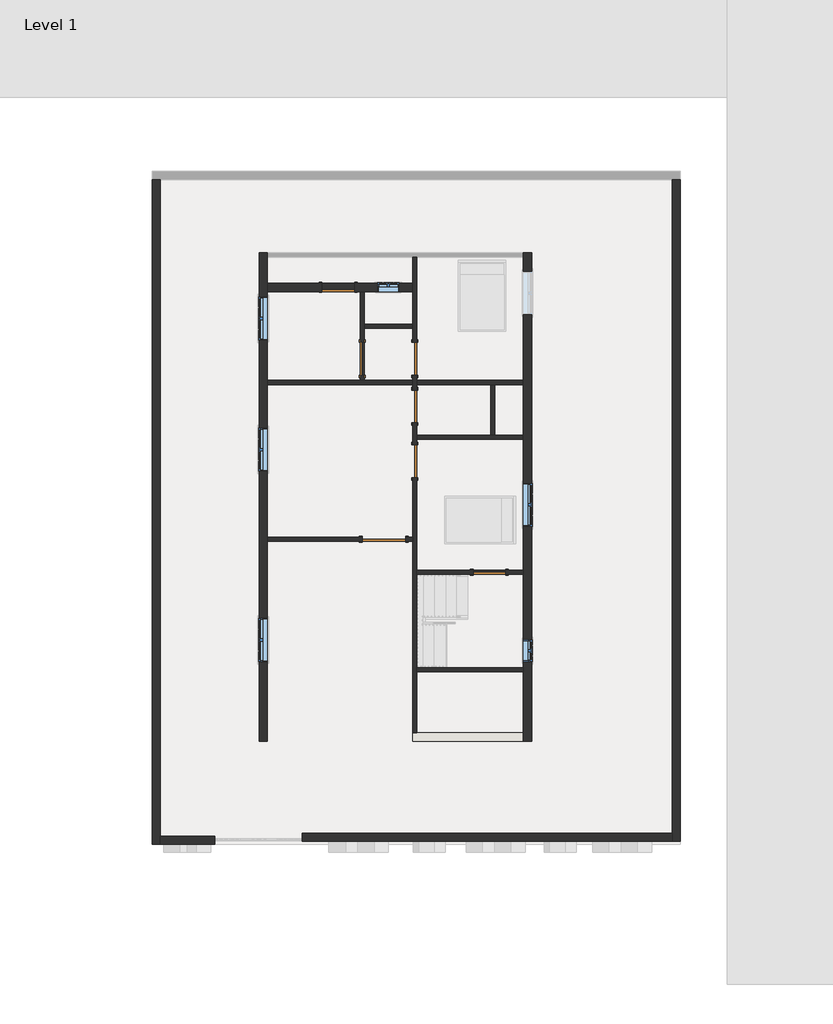
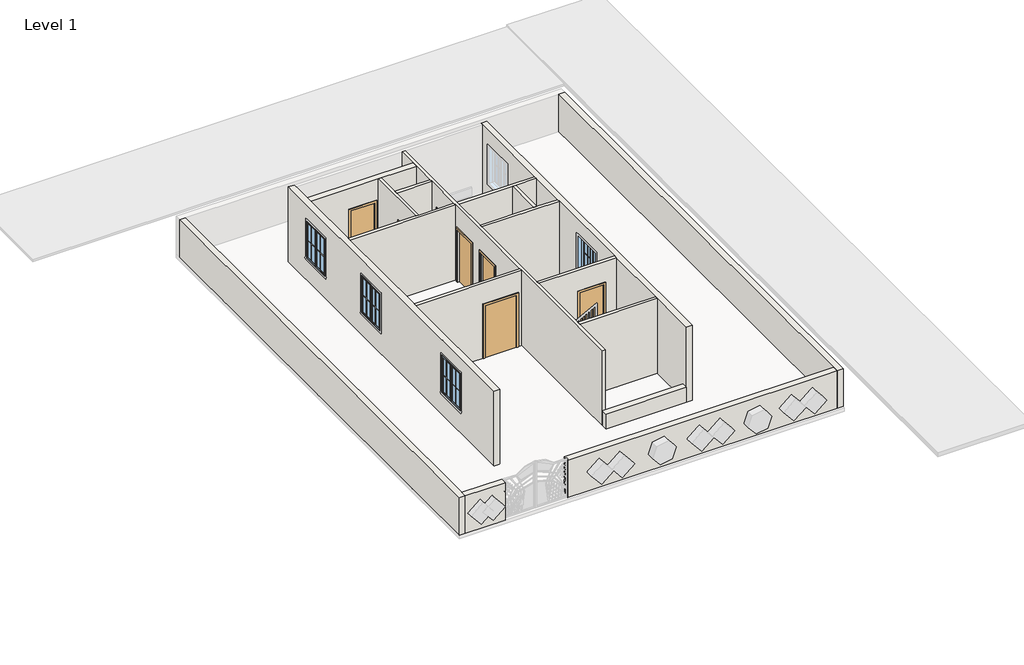
# One storey, part 1 of 7: 26 walls, 7 doors, 7 windows.
"""IFC4 building model written with IfcOpenShell, lengths in millimetres."""

from ifc_helpers import new_model, si_unit, frame, origin, origin_with_axes, place, context, project, spatial, polyline, outline, extrude, faceted_brep, transform, mapped, element, save
from components import door_a90ba1ad, door_e5f9f3c4, door_305aa2a5, door_6ea84ebe, window_c417fced, window_8377141f

model = new_model("IFC4")

# Units and contexts
model_context = context("Model", 3, world=origin())
ifc_project = project(units=[si_unit("LENGTHUNIT", "METRE", prefix="MILLI")], contexts=[model_context])

# Site, building, storey
site = spatial("IfcSite", under=ifc_project)
building = spatial("IfcBuilding", under=site)
storey = spatial("IfcBuildingStorey", under=building, Name="Level 1", Elevation=0.0)

# Doors
placement = place(None, origin())
door_shape = door_a90ba1ad(model_context)
element("IfcDoor", 1, ObjectType="Single-Flush : 36\" x 84\"", at=placement, inside=storey, context=model_context, shape_type="MappedRepresentation", body=[
    mapped(door_shape, transform((3479.8, 13512.8, 0.0), x_axis=(1.0, 0.0, 0.0), y_axis=(0.0, 1.0, 0.0), z_axis=(0.0, 0.0, 1.0))),
])
door_2_shape = door_e5f9f3c4(model_context)
element("IfcDoor", 2, ObjectType="Single-Flush : 36\" x 84\"", at=placement, inside=storey, context=model_context, shape_type="MappedRepresentation", body=[
    mapped(door_2_shape, transform((5619.75, 11518.9, 0.0), x_axis=(0.0, -1.0, 0.0), y_axis=(1.0, 0.0, 0.0), z_axis=(0.0, 0.0, 1.0))),
])
element("IfcDoor", 3, ObjectType="Single-Flush : 36\" x 84\"", at=placement, inside=storey, context=model_context, shape_type="MappedRepresentation", body=[
    mapped(door_2_shape, transform((7708.9, 5543.55, 0.0), x_axis=(-1.0, 0.0, 0.0), y_axis=(0.0, -1.0, 0.0), z_axis=(0.0, 0.0, 1.0))),
])
door_3_shape = door_305aa2a5(model_context)
element("IfcDoor", 4, ObjectType="Single-Flush : 36\" x 84\"", at=placement, inside=storey, context=model_context, shape_type="MappedRepresentation", body=[
    mapped(door_3_shape, transform((4146.55, 11518.9, 0.0), x_axis=(0.0, -1.0, 0.0), y_axis=(1.0, 0.0, 0.0), z_axis=(0.0, 0.0, 1.0))),
])
element("IfcDoor", 5, ObjectType="Single-Flush : 36\" x 84\"", at=placement, inside=storey, context=model_context, shape_type="MappedRepresentation", body=[
    mapped(door_3_shape, transform((5619.75, 10185.4, 0.0), x_axis=(0.0, 1.0, 0.0), y_axis=(-1.0, 0.0, 0.0), z_axis=(0.0, 0.0, 1.0))),
])
element("IfcDoor", 6, ObjectType="Single-Flush : 36\" x 84\"", at=placement, inside=storey, context=model_context, shape_type="MappedRepresentation", body=[
    mapped(door_3_shape, transform((5619.75, 8648.7, 0.0), x_axis=(0.0, 1.0, 0.0), y_axis=(-1.0, 0.0, 0.0), z_axis=(0.0, 0.0, 1.0))),
])
door_4_shape = door_6ea84ebe(model_context)
element("IfcDoor", 7, ObjectType="Single-Flush : 48\" x 84\"", at=placement, inside=storey, context=model_context, shape_type="MappedRepresentation", body=[
    mapped(door_4_shape, transform((4756.15, 6470.65, 0.0), x_axis=(-1.0, 0.0, 0.0), y_axis=(0.0, -1.0, 0.0), z_axis=(0.0, 0.0, 1.0))),
])

# Walls
element("IfcWall", 8, ObjectType="Generic - 5\"", at=placement, inside=storey, context=model_context, shape_type="Brep", body=[
    faceted_brep([(5562.6, 9728.2, 0.0), (5562.6, 9105.9, 0.0), (5562.6, 9105.9, 2133.6), (5562.6, 8191.5, 2133.6), (5562.6, 8191.5, 0.0), (5562.6, 6527.8, 0.0), (5562.6, 6413.5, 0.0), (5562.6, 1047.75, 0.0), (5562.6, 1047.75, 609.6), (5562.6, 1047.75, 3048.0), (5562.6, 6413.5, 3048.0), (5562.6, 6527.8, 3048.0), (5562.6, 10795.0, 3048.0), (5562.6, 10909.3, 3048.0), (5562.6, 12369.8, 3048.0), (5562.6, 12484.1, 3048.0), (5562.6, 13398.5, 3048.0), (5562.6, 13627.1, 3048.0), (5562.6, 14363.7, 3048.0), (5562.6, 14363.7, 0.0), (5562.6, 13627.1, 0.0), (5562.6, 13398.5, 0.0), (5562.6, 12484.1, 0.0), (5562.6, 12369.8, 0.0), (5562.6, 11976.1, 0.0), (5562.6, 11976.1, 2133.6), (5562.6, 11061.7, 2133.6), (5562.6, 11061.7, 0.0), (5562.6, 10909.3, 0.0), (5562.6, 10795.0, 0.0), (5562.6, 10642.6, 0.0), (5562.6, 10642.6, 2133.6), (5562.6, 9728.2, 2133.6), (5676.9, 9105.9, 2133.6), (5676.9, 9105.9, 0.0), (5676.9, 9258.3, 0.0), (5676.9, 9372.6, 0.0), (5676.9, 9728.2, 0.0), (5676.9, 9728.2, 2133.6), (5676.9, 10642.6, 2133.6), (5676.9, 10642.6, 0.0), (5676.9, 10795.0, 0.0), (5676.9, 10909.3, 0.0), (5676.9, 11061.7, 0.0), (5676.9, 11061.7, 2133.6), (5676.9, 11976.1, 2133.6), (5676.9, 11976.1, 0.0), (5676.9, 14363.7, 0.0), (5676.9, 14363.7, 3048.0), (5676.9, 10909.3, 3048.0), (5676.9, 10795.0, 3048.0), (5676.9, 9372.6, 3048.0), (5676.9, 9258.3, 3048.0), (5676.9, 5600.7, 3048.0), (5676.9, 5486.4, 3048.0), (5676.9, 2870.2, 3048.0), (5676.9, 2755.9, 3048.0), (5676.9, 1047.75, 3048.0), (5676.9, 1047.75, 0.0), (5676.9, 2755.9, 0.0), (5676.9, 2870.2, 0.0), (5676.9, 5486.4, 0.0), (5676.9, 5600.7, 0.0), (5676.9, 8191.5, 0.0), (5676.9, 8191.5, 2133.6)], [[[0, 1, 2, 3, 4, 5, 6, 7, 8, 9, 10, 11, 12, 13, 14, 15, 16, 17, 18, 19, 20, 21, 22, 23, 24, 25, 26, 27, 28, 29, 30, 31, 32]], [[33, 34, 35, 36, 37, 38, 39, 40, 41, 42, 43, 44, 45, 46, 47, 48, 49, 50, 51, 52, 53, 54, 55, 56, 57, 58, 59, 60, 61, 62, 63, 64]], [[24, 23, 22, 21, 20, 19, 47, 46]], [[43, 42, 41, 40, 30, 29, 28, 27]], [[37, 36, 35, 34, 1, 0]], [[63, 62, 61, 60, 59, 58, 7, 6, 5, 4]], [[18, 17, 16, 15, 14, 13, 12, 11, 10, 9, 57, 56, 55, 54, 53, 52, 51, 50, 49, 48]], [[19, 18, 48, 47]], [[44, 43, 27, 26]], [[45, 44, 26, 25]], [[46, 45, 25, 24]], [[31, 30, 40, 39]], [[32, 31, 39, 38]], [[0, 32, 38, 37]], [[2, 1, 34, 33]], [[3, 2, 33, 64]], [[4, 3, 64, 63]], [[9, 8, 7, 58, 57]]]),
])
element("IfcWall", 9, ObjectType="Generic - 5\"", at=placement, inside=storey, context=model_context, shape_type="SweptSolid", body=[
    extrude(outline(polyline([(0.0, 5676.9), (0.0, 7251.7), (2133.6, 7251.7), (2133.6, 8166.1), (0.0, 8166.1), (0.0, 8661.4), (3048.0, 8661.4), (3048.0, 5676.9), (0.0, 5676.9)])), frame((0.0, 5486.4, 0.0), z_axis=(0.0, 1.0, 0.0), x_axis=(0.0, 0.0, 1.0)), (0.0, 0.0, 1.0), 114.3),
])
element("IfcWall", 10, ObjectType="Generic - 5\"", at=placement, inside=storey, context=model_context, shape_type="SweptSolid", body=[
    extrude(outline(polyline([(0.0, 1498.6), (0.0, 4146.55), (2133.6, 4146.55), (2133.6, 5365.75), (0.0, 5365.75), (0.0, 5562.6), (3048.0, 5562.6), (3048.0, 1498.6), (0.0, 1498.6)])), frame((0.0, 6413.5, 0.0), z_axis=(0.0, 1.0, 0.0), x_axis=(0.0, 0.0, 1.0)), (0.0, 0.0, 1.0), 114.3),
])
element("IfcWall", 11, ObjectType="Generic - 5\"", at=placement, inside=storey, context=model_context, shape_type="Brep", body=[
    faceted_brep([(1498.6, 10795.0, 0.0), (5562.6, 10795.0, 0.0), (5562.6, 10795.0, 3048.0), (1498.6, 10795.0, 3048.0), (1498.6, 10909.3, 0.0), (1498.6, 10909.3, 3048.0), (4089.4, 10909.3, 3048.0), (4203.7, 10909.3, 3048.0), (5562.6, 10909.3, 3048.0), (5562.6, 10909.3, 0.0), (4203.7, 10909.3, 0.0), (4089.4, 10909.3, 0.0)], [[[0, 1, 2, 3]], [[4, 5, 6, 7, 8, 9, 10, 11]], [[1, 0, 4, 11, 10, 9]], [[3, 2, 8, 7, 6, 5]], [[0, 3, 5, 4]], [[2, 1, 9, 8]]]),
])
element("IfcWall", 12, ObjectType="Generic - 5\"", at=placement, inside=storey, context=model_context, shape_type="Brep", body=[
    faceted_brep([(5676.9, 10795.0, 0.0), (7747.0010433, 10795.0, 0.0), (7861.3010433, 10795.0, 0.0), (8661.4, 10795.0, 0.0), (8661.4, 10795.0, 3048.0), (7861.3010433, 10795.0, 3048.0), (7747.0010433, 10795.0, 3048.0), (5676.9, 10795.0, 3048.0), (5676.9, 10909.3, 0.0), (5676.9, 10909.3, 3048.0), (8661.4, 10909.3, 3048.0), (8661.4, 10909.3, 0.0)], [[[0, 1, 2, 3, 4, 5, 6, 7]], [[8, 9, 10, 11]], [[3, 2, 1, 0, 8, 11]], [[7, 6, 5, 4, 10, 9]], [[4, 3, 11, 10]], [[0, 7, 9, 8]]]),
])
element("IfcWall", 13, ObjectType="Generic - 5\"", at=placement, inside=storey, context=model_context, shape_type="SweptSolid", body=[
    extrude(outline(polyline([(7747.0010433, 9372.6), (7747.0010433, 10795.0), (7861.3010433, 10795.0), (7861.3010433, 9372.6), (7747.0010433, 9372.6)])), origin_with_axes(), (0.0, 0.0, 1.0), 3048.0),
])
element("IfcWall", 14, ObjectType="Generic - 5\"", at=placement, inside=storey, context=model_context, shape_type="Brep", body=[
    faceted_brep([(5676.9, 9258.3, 0.0), (8661.4, 9258.3, 0.0), (8661.4, 9258.3, 3048.0), (5676.9, 9258.3, 3048.0), (5676.9, 9372.6, 0.0), (5676.9, 9372.6, 3048.0), (7747.0010433, 9372.6, 3048.0), (7861.3010433, 9372.6, 3048.0), (8661.4, 9372.6, 3048.0), (8661.4, 9372.6, 0.0), (7861.3010433, 9372.6, 0.0), (7747.0010433, 9372.6, 0.0)], [[[0, 1, 2, 3]], [[4, 5, 6, 7, 8, 9, 10, 11]], [[1, 0, 4, 11, 10, 9]], [[3, 2, 8, 7, 6, 5]], [[2, 1, 9, 8]], [[0, 3, 5, 4]]]),
])
element("IfcWall", 15, ObjectType="Generic - 5\"", at=placement, inside=storey, context=model_context, shape_type="SweptSolid", body=[
    extrude(outline(polyline([(8661.4, 2755.9), (5676.9, 2755.9), (5676.9, 2870.2), (8661.4, 2870.2), (8661.4, 2755.9)])), origin_with_axes(), (0.0, 0.0, 1.0), 3048.0),
])
element("IfcWall", 16, ObjectType="Generic - 5\"", at=placement, inside=storey, context=model_context, shape_type="Brep", body=[
    faceted_brep([(4203.7, 10909.3, 0.0), (4203.7, 11061.7, 0.0), (4203.7, 11061.7, 2133.6), (4203.7, 11976.1, 2133.6), (4203.7, 11976.1, 0.0), (4203.7, 12369.8, 0.0), (4203.7, 12484.1, 0.0), (4203.7, 13398.5, 0.0), (4203.7, 13398.5, 3048.0), (4203.7, 12484.1, 3048.0), (4203.7, 12369.8, 3048.0), (4203.7, 10909.3, 3048.0), (4089.4, 11061.7, 2133.6), (4089.4, 11061.7, 0.0), (4089.4, 10909.3, 0.0), (4089.4, 10909.3, 3048.0), (4089.4, 13398.5, 3048.0), (4089.4, 13398.5, 0.0), (4089.4, 11976.1, 0.0), (4089.4, 11976.1, 2133.6)], [[[0, 1, 2, 3, 4, 5, 6, 7, 8, 9, 10, 11]], [[12, 13, 14, 15, 16, 17, 18, 19]], [[18, 17, 7, 6, 5, 4]], [[14, 13, 1, 0]], [[11, 10, 9, 8, 16, 15]], [[0, 11, 15, 14]], [[8, 7, 17, 16]], [[2, 1, 13, 12]], [[3, 2, 12, 19]], [[4, 3, 19, 18]]]),
])
element("IfcWall", 17, ObjectType="Generic - 5\"", at=placement, inside=storey, context=model_context, shape_type="SweptSolid", body=[
    extrude(outline(polyline([(5562.6, 12369.8), (4203.7, 12369.8), (4203.7, 12484.1), (5562.6, 12484.1), (5562.6, 12369.8)])), origin_with_axes(), (0.0, 0.0, 1.0), 3048.0),
])
element("IfcWall", 18, ObjectType="Generic - 5\"", at=placement, inside=storey, context=model_context, shape_type="SweptSolid", body=[
    extrude(outline(polyline([(8661.4, 5486.4), (5676.9, 5486.4), (5676.9, 5600.7), (8661.4, 5600.7), (8661.4, 5486.4)])), origin_with_axes(), (0.0, 0.0, 1.0), 3048.0),
])
element("IfcWall", 19, ObjectType="Generic - 5\"", at=placement, inside=storey, context=model_context, shape_type="Brep", body=[
    faceted_brep([(1498.6, 10795.0, 0.0), (5562.6, 10795.0, 0.0), (5562.6, 10795.0, 3048.0), (1498.6, 10795.0, 3048.0), (1498.6, 10909.3, 0.0), (1498.6, 10909.3, 3048.0), (4089.4, 10909.3, 3048.0), (4203.7, 10909.3, 3048.0), (5562.6, 10909.3, 3048.0), (5562.6, 10909.3, 0.0), (4203.7, 10909.3, 0.0), (4089.4, 10909.3, 0.0)], [[[0, 1, 2, 3]], [[4, 5, 6, 7, 8, 9, 10, 11]], [[1, 0, 4, 11, 10, 9]], [[3, 2, 8, 7, 6, 5]], [[0, 3, 5, 4]], [[2, 1, 9, 8]]]),
])
element("IfcWall", 20, ObjectType="Generic - 5\"", at=placement, inside=storey, context=model_context, shape_type="Brep", body=[
    faceted_brep([(5676.9, 10795.0, 0.0), (7747.0010433, 10795.0, 0.0), (7861.3010433, 10795.0, 0.0), (8661.4, 10795.0, 0.0), (8661.4, 10795.0, 3048.0), (7861.3010433, 10795.0, 3048.0), (7747.0010433, 10795.0, 3048.0), (5676.9, 10795.0, 3048.0), (5676.9, 10909.3, 0.0), (5676.9, 10909.3, 3048.0), (8661.4, 10909.3, 3048.0), (8661.4, 10909.3, 0.0)], [[[0, 1, 2, 3, 4, 5, 6, 7]], [[8, 9, 10, 11]], [[3, 2, 1, 0, 8, 11]], [[7, 6, 5, 4, 10, 9]], [[4, 3, 11, 10]], [[0, 7, 9, 8]]]),
])
element("IfcWall", 21, ObjectType="Generic - 5\"", at=placement, inside=storey, context=model_context, shape_type="SweptSolid", body=[
    extrude(outline(polyline([(7747.0010433, 9372.6), (7747.0010433, 10795.0), (7861.3010433, 10795.0), (7861.3010433, 9372.6), (7747.0010433, 9372.6)])), origin_with_axes(), (0.0, 0.0, 1.0), 3048.0),
])
element("IfcWall", 22, ObjectType="Generic - 5\"", at=placement, inside=storey, context=model_context, shape_type="Brep", body=[
    faceted_brep([(5676.9, 9258.3, 0.0), (8661.4, 9258.3, 0.0), (8661.4, 9258.3, 3048.0), (5676.9, 9258.3, 3048.0), (5676.9, 9372.6, 0.0), (5676.9, 9372.6, 3048.0), (7747.0010433, 9372.6, 3048.0), (7861.3010433, 9372.6, 3048.0), (8661.4, 9372.6, 3048.0), (8661.4, 9372.6, 0.0), (7861.3010433, 9372.6, 0.0), (7747.0010433, 9372.6, 0.0)], [[[0, 1, 2, 3]], [[4, 5, 6, 7, 8, 9, 10, 11]], [[1, 0, 4, 11, 10, 9]], [[3, 2, 8, 7, 6, 5]], [[2, 1, 9, 8]], [[0, 3, 5, 4]]]),
])
element("IfcWall", 23, ObjectType="Generic - 5\"", at=placement, inside=storey, context=model_context, shape_type="Brep", body=[
    faceted_brep([(4203.7, 10909.3, 0.0), (4203.7, 12369.8, 0.0), (4203.7, 12484.1, 0.0), (4203.7, 13398.5, 0.0), (4203.7, 13398.5, 3048.0), (4203.7, 12484.1, 3048.0), (4203.7, 12369.8, 3048.0), (4203.7, 10909.3, 3048.0), (4089.4, 10909.3, 0.0), (4089.4, 10909.3, 3048.0), (4089.4, 13398.5, 3048.0), (4089.4, 13398.5, 0.0)], [[[0, 1, 2, 3, 4, 5, 6, 7]], [[8, 9, 10, 11]], [[3, 2, 1, 0, 8, 11]], [[7, 6, 5, 4, 10, 9]], [[0, 7, 9, 8]], [[4, 3, 11, 10]]]),
])
element("IfcWall", 24, ObjectType="Generic - 5\"", at=placement, inside=storey, context=model_context, shape_type="SweptSolid", body=[
    extrude(outline(polyline([(5562.6, 12369.8), (4203.7, 12369.8), (4203.7, 12484.1), (5562.6, 12484.1), (5562.6, 12369.8)])), origin_with_axes(), (0.0, 0.0, 1.0), 3048.0),
])
element("IfcWall", 25, ObjectType="Generic - 8\"", at=placement, inside=storey, context=model_context, shape_type="Brep", body=[
    faceted_brep([(8661.4, 14478.0, 0.0), (8661.4, 14363.7, 0.0), (8661.4, 10909.3, 0.0), (8661.4, 10795.0, 0.0), (8661.4, 9372.6, 0.0), (8661.4, 9258.3, 0.0), (8661.4, 5600.7, 0.0), (8661.4, 5486.4, 0.0), (8661.4, 2870.2, 0.0), (8661.4, 2755.9, 0.0), (8661.4, 1047.75, 0.0), (8661.4, 819.15, 0.0), (8661.4, 819.15, 609.6), (8661.4, 819.15, 3048.0), (8661.4, 2755.9, 3048.0), (8661.4, 2870.2, 3048.0), (8661.4, 5486.4, 3048.0), (8661.4, 5600.7, 3048.0), (8661.4, 9258.3, 3048.0), (8661.4, 9372.6, 3048.0), (8661.4, 10795.0, 3048.0), (8661.4, 10909.3, 3048.0), (8661.4, 14363.7, 3048.0), (8661.4, 14478.0, 3048.0), (8661.4, 6819.9, 2438.4), (8661.4, 6819.9, 914.4), (8661.4, 8039.1, 914.4), (8661.4, 8039.1, 2438.4), (8661.4, 12744.45, 2438.4), (8661.4, 12744.45, 914.4), (8661.4, 13963.65, 914.4), (8661.4, 13963.65, 2438.4), (8661.4, 3041.65, 1828.8), (8661.4, 3041.65, 914.4), (8661.4, 3651.25, 914.4), (8661.4, 3651.25, 1828.8), (8890.0, 14478.0, 0.0), (8890.0, 14478.0, 3048.0), (8890.0, 819.15, 3048.0), (8890.0, 819.15, 0.0), (8890.0, 6819.9, 2438.4), (8890.0, 8039.1, 2438.4), (8890.0, 8039.1, 914.4), (8890.0, 6819.9, 914.4), (8890.0, 12744.45, 2438.4), (8890.0, 13963.65, 2438.4), (8890.0, 13963.65, 914.4), (8890.0, 12744.45, 914.4), (8890.0, 3041.65, 1828.8), (8890.0, 3651.25, 1828.8), (8890.0, 3651.25, 914.4), (8890.0, 3041.65, 914.4)], [[[0, 1, 2, 3, 4, 5, 6, 7, 8, 9, 10, 11, 12, 13, 14, 15, 16, 17, 18, 19, 20, 21, 22, 23], [24, 25, 26, 27], [28, 29, 30, 31], [32, 33, 34, 35]], [[36, 37, 38, 39], [40, 41, 42, 43], [44, 45, 46, 47], [48, 49, 50, 51]], [[11, 10, 9, 8, 7, 6, 5, 4, 3, 2, 1, 0, 36, 39]], [[23, 22, 21, 20, 19, 18, 17, 16, 15, 14, 13, 38, 37]], [[0, 23, 37, 36]], [[25, 24, 40, 43]], [[26, 25, 43, 42]], [[27, 26, 42, 41]], [[24, 27, 41, 40]], [[29, 28, 44, 47]], [[30, 29, 47, 46]], [[31, 30, 46, 45]], [[28, 31, 45, 44]], [[33, 32, 48, 51]], [[34, 33, 51, 50]], [[35, 34, 50, 49]], [[32, 35, 49, 48]], [[13, 12, 11, 39, 38]]]),
])
element("IfcWall", 26, ObjectType="Generic - 8\"", at=placement, inside=storey, context=model_context, shape_type="Brep", body=[
    faceted_brep([(1270.0, 14478.0, 0.0), (1270.0, 819.15, 0.0), (1270.0, 819.15, 3048.0), (1270.0, 14478.0, 3048.0), (1270.0, 9582.15, 2438.4), (1270.0, 8362.95, 2438.4), (1270.0, 8362.95, 914.4), (1270.0, 9582.15, 914.4), (1270.0, 4254.5, 2438.4), (1270.0, 3035.3, 2438.4), (1270.0, 3035.3, 914.4), (1270.0, 4254.5, 914.4), (1270.0, 13252.45, 2438.4), (1270.0, 12033.25, 2438.4), (1270.0, 12033.25, 914.4), (1270.0, 13252.45, 914.4), (1498.6, 14478.0, 0.0), (1498.6, 14478.0, 3048.0), (1498.6, 14363.7, 3048.0), (1498.6, 13627.1, 3048.0), (1498.6, 13398.5, 3048.0), (1498.6, 10909.3, 3048.0), (1498.6, 10795.0, 3048.0), (1498.6, 6527.8, 3048.0), (1498.6, 6413.5, 3048.0), (1498.6, 819.15, 3048.0), (1498.6, 819.15, 0.0), (1498.6, 6413.5, 0.0), (1498.6, 6527.8, 0.0), (1498.6, 10795.0, 0.0), (1498.6, 10909.3, 0.0), (1498.6, 13398.5, 0.0), (1498.6, 13627.1, 0.0), (1498.6, 14363.7, 0.0), (1498.6, 9582.15, 2438.4), (1498.6, 9582.15, 914.4), (1498.6, 8362.95, 914.4), (1498.6, 8362.95, 2438.4), (1498.6, 4254.5, 2438.4), (1498.6, 4254.5, 914.4), (1498.6, 3035.3, 914.4), (1498.6, 3035.3, 2438.4), (1498.6, 13252.45, 2438.4), (1498.6, 13252.45, 914.4), (1498.6, 12033.25, 914.4), (1498.6, 12033.25, 2438.4)], [[[0, 1, 2, 3], [4, 5, 6, 7], [8, 9, 10, 11], [12, 13, 14, 15]], [[16, 17, 18, 19, 20, 21, 22, 23, 24, 25, 26, 27, 28, 29, 30, 31, 32, 33], [34, 35, 36, 37], [38, 39, 40, 41], [42, 43, 44, 45]], [[1, 0, 16, 33, 32, 31, 30, 29, 28, 27, 26]], [[2, 1, 26, 25]], [[3, 2, 25, 24, 23, 22, 21, 20, 19, 18, 17]], [[0, 3, 17, 16]], [[35, 34, 4, 7]], [[36, 35, 7, 6]], [[37, 36, 6, 5]], [[34, 37, 5, 4]], [[39, 38, 8, 11]], [[40, 39, 11, 10]], [[41, 40, 10, 9]], [[38, 41, 9, 8]], [[43, 42, 12, 15]], [[44, 43, 15, 14]], [[45, 44, 14, 13]], [[42, 45, 13, 12]]]),
])
element("IfcWall", 27, ObjectType="Generic - 8\"", at=placement, inside=storey, context=model_context, shape_type="Brep", body=[
    faceted_brep([(3937.0, 13398.5, 2133.6), (3937.0, 13398.5, 0.0), (4089.4, 13398.5, 0.0), (4203.7, 13398.5, 0.0), (5562.6, 13398.5, 0.0), (5562.6, 13398.5, 3048.0), (4203.7, 13398.5, 3048.0), (4089.4, 13398.5, 3048.0), (1498.6, 13398.5, 3048.0), (1498.6, 13398.5, 0.0), (3022.6, 13398.5, 0.0), (3022.6, 13398.5, 2133.6), (5187.95, 13398.5, 1828.8), (5187.95, 13398.5, 914.4), (4578.35, 13398.5, 914.4), (4578.35, 13398.5, 1828.8), (5562.6, 13627.1, 0.0), (3937.0, 13627.1, 0.0), (3937.0, 13627.1, 2133.6), (3022.6, 13627.1, 2133.6), (3022.6, 13627.1, 0.0), (1498.6, 13627.1, 0.0), (1498.6, 13627.1, 3048.0), (5562.6, 13627.1, 3048.0), (5187.95, 13627.1, 1828.8), (4578.35, 13627.1, 1828.8), (4578.35, 13627.1, 914.4), (5187.95, 13627.1, 914.4)], [[[0, 1, 2, 3, 4, 5, 6, 7, 8, 9, 10, 11], [12, 13, 14, 15]], [[16, 17, 18, 19, 20, 21, 22, 23], [24, 25, 26, 27]], [[10, 9, 21, 20]], [[4, 3, 2, 1, 17, 16]], [[8, 7, 6, 5, 23, 22]], [[9, 8, 22, 21]], [[5, 4, 16, 23]], [[18, 17, 1, 0]], [[19, 18, 0, 11]], [[20, 19, 11, 10]], [[13, 12, 24, 27]], [[14, 13, 27, 26]], [[15, 14, 26, 25]], [[12, 15, 25, 24]]]),
])
element("IfcWall", 28, ObjectType="Generic - 8\"", at=placement, inside=storey, context=model_context, shape_type="Brep", body=[
    faceted_brep([(1498.6, 13398.5, 0.0), (4089.4, 13398.5, 0.0), (4203.7, 13398.5, 0.0), (5562.6, 13398.5, 0.0), (5562.6, 13398.5, 3048.0), (4203.7, 13398.5, 3048.0), (4089.4, 13398.5, 3048.0), (1498.6, 13398.5, 3048.0), (5187.95, 13398.5, 1828.8), (5187.95, 13398.5, 914.4), (4578.35, 13398.5, 914.4), (4578.35, 13398.5, 1828.8), (1498.6, 13627.1, 0.0), (1498.6, 13627.1, 3048.0), (5562.6, 13627.1, 3048.0), (5562.6, 13627.1, 0.0), (5187.95, 13627.1, 1828.8), (4578.35, 13627.1, 1828.8), (4578.35, 13627.1, 914.4), (5187.95, 13627.1, 914.4)], [[[0, 1, 2, 3, 4, 5, 6, 7], [8, 9, 10, 11]], [[12, 13, 14, 15], [16, 17, 18, 19]], [[3, 2, 1, 0, 12, 15]], [[7, 6, 5, 4, 14, 13]], [[9, 8, 16, 19]], [[10, 9, 19, 18]], [[11, 10, 18, 17]], [[8, 11, 17, 16]], [[0, 7, 13, 12]], [[4, 3, 15, 14]]]),
])
element("IfcWall", 29, ObjectType="Generic - 8\"", at=placement, inside=storey, context=model_context, shape_type="Brep", body=[
    faceted_brep([(12827.9234142, 16532.995404, 0.0), (12827.9234142, -1755.004596, 0.0), (12827.9234142, -1983.604596, 0.0), (12827.9234142, -1983.604596, 1524.0), (12827.9234142, -1755.004596, 1524.0), (12827.9234142, 16532.995404, 1524.0), (13056.5234142, 16532.995404, 0.0), (13056.5234142, 16532.995404, 1524.0), (13056.5234142, -1983.604596, 1524.0), (13056.5234142, -1983.604596, 0.0)], [[[0, 1, 2, 3, 4, 5]], [[6, 7, 8, 9]], [[2, 1, 0, 6, 9]], [[5, 4, 3, 8, 7]], [[0, 5, 7, 6]], [[3, 2, 9, 8]]]),
])
element("IfcWall", 30, ObjectType="Generic - 8\"", at=placement, inside=storey, context=model_context, shape_type="SweptSolid", body=[
    extrude(outline(polyline([(2477.4234142, -1755.004596), (12827.9234142, -1755.004596), (12827.9234142, -1983.604596), (2477.4234142, -1983.604596), (2477.4234142, -1755.004596)])), origin_with_axes(), (0.0, 0.0, 1.0), 1524.0),
])
element("IfcWall", 31, ObjectType="Generic - 8\"", at=placement, inside=storey, context=model_context, shape_type="Brep", body=[
    faceted_brep([(-1497.6765858, -2075.0517987, 0.0), (-1497.6765858, -1846.4517987, 0.0), (-1497.6765858, 16532.995404, 0.0), (-1497.6765858, 16532.995404, 1524.0), (-1497.6765858, -1846.4517987, 1524.0), (-1497.6765858, -2075.0517987, 1524.0), (-1726.2765858, -2075.0517987, 0.0), (-1726.2765858, -2075.0517987, 1524.0), (-1726.2765858, 16532.995404, 1524.0), (-1726.2765858, 16532.995404, 0.0)], [[[0, 1, 2, 3, 4, 5]], [[6, 7, 8, 9]], [[2, 1, 0, 6, 9]], [[5, 4, 3, 8, 7]], [[3, 2, 9, 8]], [[0, 5, 7, 6]]]),
])
element("IfcWall", 32, ObjectType="Generic - 8\"", at=placement, inside=storey, context=model_context, shape_type="SweptSolid", body=[
    extrude(outline(polyline([(-1497.6765858, -1846.4517987), (26.2511206, -1846.4517987), (26.2511206, -2075.0517987), (-1497.6765858, -2075.0517987), (-1497.6765858, -1846.4517987)])), origin_with_axes(), (0.0, 0.0, 1.0), 1524.0),
])
element("IfcWall", 33, ObjectType="Generic - 8\"", at=placement, inside=storey, context=model_context, shape_type="Brep", body=[
    faceted_brep([(8661.4, 1047.75, 0.0), (5676.9, 1047.75, 0.0), (5562.6, 1047.75, 0.0), (5562.6, 1047.75, 609.6), (8661.4, 1047.75, 609.6), (8661.4, 819.15, 0.0), (8661.4, 819.15, 609.6), (5562.6, 819.15, 609.6), (5562.6, 819.15, 0.0)], [[[0, 1, 2, 3, 4]], [[5, 6, 7, 8]], [[2, 1, 0, 5, 8]], [[4, 3, 7, 6]], [[0, 4, 6, 5]], [[3, 2, 8, 7]]]),
])

# Windows
window_shape = window_c417fced(model_context)
element("IfcWindow", 34, ObjectType="Window-Casement-Double : 24\" x 36\"", at=placement, inside=storey, context=model_context, shape_type="MappedRepresentation", body=[
    mapped(window_shape, transform((4883.15, 13512.8, 0.0), x_axis=(1.0, 0.0, 0.0), y_axis=(0.0, 1.0, 0.0), z_axis=(0.0, 0.0, 1.0))),
])
element("IfcWindow", 35, ObjectType="Window-Casement-Double : 24\" x 36\"", at=placement, inside=storey, context=model_context, shape_type="MappedRepresentation", body=[
    mapped(window_shape, transform((8775.7, 3346.45, 0.0), x_axis=(0.0, -1.0, 0.0), y_axis=(1.0, 0.0, 0.0), z_axis=(0.0, 0.0, 1.0))),
])
element("IfcWindow", 36, ObjectType="Window-Casement-Double : 24\" x 36\"", at=placement, inside=storey, context=model_context, shape_type="MappedRepresentation", body=[
    mapped(window_shape, transform((4883.15, 13512.8, 0.0), x_axis=(1.0, 0.0, 0.0), y_axis=(0.0, 1.0, 0.0), z_axis=(0.0, 0.0, 1.0))),
])
window_2_shape = window_8377141f(model_context)
element("IfcWindow", 37, ObjectType="Window-Casement-Double : 48\" x 60\"", at=placement, inside=storey, context=model_context, shape_type="MappedRepresentation", body=[
    mapped(window_2_shape, transform((1384.3, 8972.55, 0.0), x_axis=(0.0, 1.0, 0.0), y_axis=(-1.0, 0.0, 0.0), z_axis=(0.0, 0.0, 1.0))),
])
element("IfcWindow", 38, ObjectType="Window-Casement-Double : 48\" x 60\"", at=placement, inside=storey, context=model_context, shape_type="MappedRepresentation", body=[
    mapped(window_2_shape, transform((1384.3, 3644.9, 0.0), x_axis=(0.0, 1.0, 0.0), y_axis=(-1.0, 0.0, 0.0), z_axis=(0.0, 0.0, 1.0))),
])
element("IfcWindow", 39, ObjectType="Window-Casement-Double : 48\" x 60\"", at=placement, inside=storey, context=model_context, shape_type="MappedRepresentation", body=[
    mapped(window_2_shape, transform((8775.7, 7429.5, 0.0), x_axis=(0.0, -1.0, 0.0), y_axis=(1.0, 0.0, 0.0), z_axis=(0.0, 0.0, 1.0))),
])
element("IfcWindow", 40, ObjectType="Window-Casement-Double : 48\" x 60\"", at=placement, inside=storey, context=model_context, shape_type="MappedRepresentation", body=[
    mapped(window_2_shape, transform((1384.3, 12642.85, 0.0), x_axis=(0.0, 1.0, 0.0), y_axis=(-1.0, 0.0, 0.0), z_axis=(0.0, 0.0, 1.0))),
])

save(model, "model.ifc")

# Revit data of these elements
# Type "Single-Flush : 36\" x 84\""
#   Type Mark = "1"
#   Construction Type Id = "MDOOR"
#   Assembly Code = "C1020"
#   Analytic Construction = "Metal"
#   Thickness = 0' - 2"
#   Heat Transfer Coefficient (U) = 0.651978 BTU/(h·ft²·°F)
#   Height = 7' - 0"
#   Trim Projection Ext = 0' - 1"
#   Trim Projection Int = 0' - 1"
#   Trim Width = 0' - 3"
#   Width = 3' - 0"
#   Define Thermal Properties by = 1
#   Define Thermal Properties by = 1
#   Door Material = Door - Panel
#   Frame Material = Door - Frame
#   Visual Light Transmittance = 0
#   Solar Heat Gain Coefficient = 0
#   Function = (empty or 0)
#   Wall Closure = (empty or 0)
# Type "Single-Flush : 48\" x 84\""
#   Type Mark = "5"
#   Construction Type Id = "MDOOR"
#   Assembly Code = "C1020"
#   Analytic Construction = "Metal"
#   Thickness = 0' - 2"
#   Heat Transfer Coefficient (U) = 0.651978 BTU/(h·ft²·°F)
#   Height = 7' - 0"
#   Trim Projection Ext = 0' - 1"
#   Trim Projection Int = 0' - 1"
#   Trim Width = 0' - 3"
#   Width = 4' - 0"
#   Define Thermal Properties by = 1
#   Define Thermal Properties by = 1
#   Door Material = Door - Panel
#   Frame Material = Door - Frame
#   Visual Light Transmittance = 0
#   Solar Heat Gain Coefficient = 0
#   Function = (empty or 0)
#   Wall Closure = (empty or 0)
# Type "Generic - 5\""
#   Assembly Code = "B2010"
#   Layers, outside or top first: 0' - 4 1/2" no material (function 1)
# Type "Generic - 8\""
#   Assembly Code = "B2010"
#   Layers, outside or top first: 0' - 9" no material (function 1)
# Type "Window-Casement-Double : 24\" x 36\""
#   Type Mark = "14"
#   Fire Rating = "0.5h"
#   Assembly Code = "B2020100"
#   Analytic Construction = "Double glazing - domestic"
#   Frame Extension [instance default] = 0' - 0 1/4"
#   Window Inset [instance default] = 0' - 0"
#   Wall Thickness [instance default] = 0' - 6"
#   Interior Wall Closure [instance default] = 0' - 2 1/4"
#   Half Width = 1' - 0"
#   Visual Light Transmittance = 0.81
#   Thermal Resistance (R) = 1.8146 (h·ft²·°F)/BTU
#   Solar Heat Gain Coefficient = 0.76
#   Rough Width = 2' - 0 1/2"
#   Rough Height = 3' - 0 1/2"
#   Height = 3' - 0"
#   Heat Transfer Coefficient (U) = 0.5511 BTU/(h·ft²·°F)
#   Exterior Wall Closure [instance default] = 0' - 1 1/4"
#   Extension Jamb [instance default] = 0' - 2 1/4"
#   Default Sill Height = 3' - 0"
#   Width = 2' - 0"
#   Define Thermal Properties by = 0
#   Muntin Visibility = yes
#   Interior Trim Visibility [instance default] = yes
#   Exterior Trim Visibility [instance default] = yes
#   Extension Jamb Visibility [instance default] = yes
#   Interior Trim Material = Wood - Stained
#   Muntin Pattern = Muntin Pattern_2x2 : Muntin Pattern_2x2
#   Interior Trim = Trim-Window-Interior-Flat : Picture Frame
#   Interior Frame Material = Wood - Stained
#   Glass Panel Material = Glass
#   Exterior Trim Material = Clad - White
#   Exterior Trim = Trim-Window-Exterior-Flat : with Sill
#   Exterior Frame Material = Clad - White
#   Wall Closure = (empty or 0)
# Type "Window-Casement-Double : 48\" x 60\""
#   Type Mark = "17"
#   Fire Rating = "0.5h"
#   Assembly Code = "B2020100"
#   Analytic Construction = "Double glazing - domestic"
#   Frame Extension [instance default] = 0' - 0 1/4"
#   Window Inset [instance default] = 0' - 0"
#   Wall Thickness [instance default] = 0' - 6"
#   Interior Wall Closure [instance default] = 0' - 2 1/4"
#   Half Width = 2' - 0"
#   Visual Light Transmittance = 0.81
#   Thermal Resistance (R) = 1.8146 (h·ft²·°F)/BTU
#   Solar Heat Gain Coefficient = 0.76
#   Rough Width = 4' - 0 1/2"
#   Rough Height = 5' - 0 1/2"
#   Height = 5' - 0"
#   Heat Transfer Coefficient (U) = 0.5511 BTU/(h·ft²·°F)
#   Exterior Wall Closure [instance default] = 0' - 1 1/4"
#   Extension Jamb [instance default] = 0' - 2 1/4"
#   Default Sill Height = 3' - 0"
#   Width = 4' - 0"
#   Define Thermal Properties by = 0
#   Muntin Visibility = yes
#   Interior Trim Visibility [instance default] = yes
#   Exterior Trim Visibility [instance default] = yes
#   Extension Jamb Visibility [instance default] = yes
#   Interior Trim Material = Wood - Stained
#   Muntin Pattern = Muntin Pattern_2x2 : Muntin Pattern_2x2
#   Interior Trim = Trim-Window-Interior-Flat : Picture Frame
#   Interior Frame Material = Wood - Stained
#   Glass Panel Material = Glass
#   Exterior Trim Material = Clad - White
#   Exterior Trim = Trim-Window-Exterior-Flat : with Sill
#   Exterior Frame Material = Clad - White
#   Wall Closure = (empty or 0)
# Elements 1, 2, 3, 4, 5, 6 (IfcDoor, "Single-Flush : 36\" x 84\"")
#   Phase Created = New Construction
#   Materials on its faces: "Door - Frame", "Door - Panel"
# Element 7 (IfcDoor, "Single-Flush : 48\" x 84\"")
#   Phase Created = New Construction
#   Materials on its faces: "Door - Frame", "Door - Panel"
# Element 8 (IfcWall, "Generic - 5\"")
#   Top Offset = 0' - 0"
#   Base Offset = 0' - 0"
#   wall height = 10' - 0"
#   Phase Created = New Construction
#   Base Constraint = Level 1
#   Top Constraint = Level 2
#   Materials on its faces: "Default Wall", "Parking Stripe", "Carpet (1)"
# Elements 9, 11, 12, 13, 14, 16, 17, 18, 19, 20, 21, 22, 23, 24 (IfcWall, "Generic - 5\"")
#   Top Offset = 0' - 0"
#   Base Offset = 0' - 0"
#   wall height = 10' - 0"
#   Phase Created = New Construction
#   Base Constraint = Level 1
#   Top Constraint = Level 2
#   Materials on its faces: "Default Wall"
# Elements 10, 15 (IfcWall, "Generic - 5\"")
#   Top Offset = 0' - 0"
#   Base Offset = 0' - 0"
#   wall height = 10' - 0"
#   Phase Created = New Construction
#   Base Constraint = Level 1
#   Top Constraint = Level 2
#   Materials on its faces: "Default Wall", "Parking Stripe"
# Element 25 (IfcWall, "Generic - 8\"")
#   Top Offset = 0' - 0"
#   Base Offset = 0' - 0"
#   Unconnected Height = 10' - 0"
#   wall height = 10' - 0"
#   Phase Created = New Construction
#   Base Constraint = Level 1
#   Materials on its faces: "Default Wall", "Parking Stripe", "Plywood, Sheathing", "Carpet (1)"
# Element 26 (IfcWall, "Generic - 8\"")
#   Top Offset = 0' - 0"
#   Base Offset = 0' - 0"
#   Unconnected Height = 10' - 0"
#   wall height = 10' - 0"
#   Phase Created = New Construction
#   Base Constraint = Level 1
#   Materials on its faces: "Default Wall", "Parking Stripe", "Carpet (1)"
# Elements 27, 28 (IfcWall, "Generic - 8\"")
#   Top Offset = 0' - 0"
#   Base Offset = 0' - 0"
#   Unconnected Height = 10' - 0"
#   wall height = 10' - 0"
#   Phase Created = New Construction
#   Base Constraint = Level 1
#   Materials on its faces: "Default Wall"
# Elements 29, 31 (IfcWall, "Generic - 8\"")
#   Top Offset = 0' - 0"
#   Base Offset = 0' - 0"
#   Unconnected Height = 5' - 0"
#   wall height = 5' - 0"
#   Phase Created = New Construction
#   Base Constraint = Level 1
#   Materials on its faces: "Door - Frame", "Default Wall", "Clad - White"
# Elements 30, 32 (IfcWall, "Generic - 8\"")
#   Top Offset = 0' - 0"
#   Base Offset = 0' - 0"
#   Unconnected Height = 5' - 0"
#   wall height = 5' - 0"
#   Phase Created = New Construction
#   Base Constraint = Level 1
#   Materials on its faces: "Default Wall", "Door - Frame", "Clad - White"
# Element 33 (IfcWall, "Generic - 8\"")
#   Top Offset = 0' - 0"
#   Base Offset = 0' - 0"
#   Unconnected Height = 2' - 0"
#   wall height = 2' - 0"
#   Phase Created = New Construction
#   Base Constraint = Level 1
#   Materials on its faces: "Default Wall", "Carpet (1)", "Parking Stripe"
# Element 34 (IfcWindow, "Window-Casement-Double : 24\" x 36\"")
#   Mark = "6"
#   Window Inset = 0' - 0"
#   Interior Wall Closure = 0' - 2 1/4"
#   Frame Extension = 0' - 0 1/4"
#   Exterior Wall Closure = 0' - 1 1/4"
#   Interior Trim Visibility = yes
#   Exterior Trim Visibility = yes
#   Phase Created = New Construction
#   Materials on its faces: "Wood - Stained", "Glass", "Clad - White"
# Element 35 (IfcWindow, "Window-Casement-Double : 24\" x 36\"")
#   Mark = "7"
#   Window Inset = 0' - 0"
#   Interior Wall Closure = 0' - 2 1/4"
#   Frame Extension = 0' - 0 1/4"
#   Exterior Wall Closure = 0' - 1 1/4"
#   Interior Trim Visibility = yes
#   Exterior Trim Visibility = yes
#   Phase Created = New Construction
#   Materials on its faces: "Wood - Stained", "Glass", "Clad - White"
# Element 36 (IfcWindow, "Window-Casement-Double : 24\" x 36\"")
#   Mark = "13"
#   Window Inset = 0' - 0"
#   Interior Wall Closure = 0' - 2 1/4"
#   Frame Extension = 0' - 0 1/4"
#   Exterior Wall Closure = 0' - 1 1/4"
#   Interior Trim Visibility = yes
#   Exterior Trim Visibility = yes
#   Phase Created = New Construction
#   Materials on its faces: "Wood - Stained", "Glass", "Clad - White"
# Element 37 (IfcWindow, "Window-Casement-Double : 48\" x 60\"")
#   Mark = "1"
#   Window Inset = 0' - 0"
#   Interior Wall Closure = 0' - 2 1/4"
#   Frame Extension = 0' - 0 1/4"
#   Exterior Wall Closure = 0' - 1 1/4"
#   Interior Trim Visibility = yes
#   Exterior Trim Visibility = yes
#   Phase Created = New Construction
#   Materials on its faces: "Wood - Stained", "Glass", "Clad - White"
# Element 38 (IfcWindow, "Window-Casement-Double : 48\" x 60\"")
#   Mark = "2"
#   Window Inset = 0' - 0"
#   Interior Wall Closure = 0' - 2 1/4"
#   Frame Extension = 0' - 0 1/4"
#   Exterior Wall Closure = 0' - 1 1/4"
#   Interior Trim Visibility = yes
#   Exterior Trim Visibility = yes
#   Phase Created = New Construction
#   Materials on its faces: "Wood - Stained", "Glass", "Clad - White"
# Element 39 (IfcWindow, "Window-Casement-Double : 48\" x 60\"")
#   Mark = "3"
#   Window Inset = 0' - 0"
#   Interior Wall Closure = 0' - 2 1/4"
#   Frame Extension = 0' - 0 1/4"
#   Exterior Wall Closure = 0' - 1 1/4"
#   Interior Trim Visibility = yes
#   Exterior Trim Visibility = yes
#   Phase Created = New Construction
#   Materials on its faces: "Wood - Stained", "Glass", "Clad - White"
# Element 40 (IfcWindow, "Window-Casement-Double : 48\" x 60\"")
#   Mark = "5"
#   Window Inset = 0' - 0"
#   Interior Wall Closure = 0' - 2 1/4"
#   Frame Extension = 0' - 0 1/4"
#   Exterior Wall Closure = 0' - 1 1/4"
#   Interior Trim Visibility = yes
#   Exterior Trim Visibility = yes
#   Phase Created = New Construction
#   Materials on its faces: "Wood - Stained", "Glass", "Clad - White"
# Materials
#   "Door - Panel": class "Wood", colour RGB 210 159 95, transparency 0, Cost = 0
#   "Door - Frame": colour RGB 118 70 51, transparency 0, Cost = 0
#   "Wood - Stained": class "Wood", colour RGB 224 178 126, transparency 0, Cost = 0
#   "Glass": class "Glass", colour RGB 0 128 192, transparency 0.75, Description = "Soda Lime Glass", Cost = 0
#   "Clad - White": class "Wood", colour RGB 242 242 238, transparency 0, Cost = 0
#   "Default Wall": colour RGB 128 128 128, transparency 0, Cost = 0
#   "Parking Stripe": class "Paint", colour RGB 250 250 91, transparency 0, Cost = 0
#   "Carpet (1)": class "Carpet", colour RGB 124 80 67, transparency 0, Description = "Interior finish", Cost = 0
#   "Plywood, Sheathing": class "Wood", colour RGB 212 179 113, transparency 0, Description = "Plywood, sheathing grade", Cost = 0
